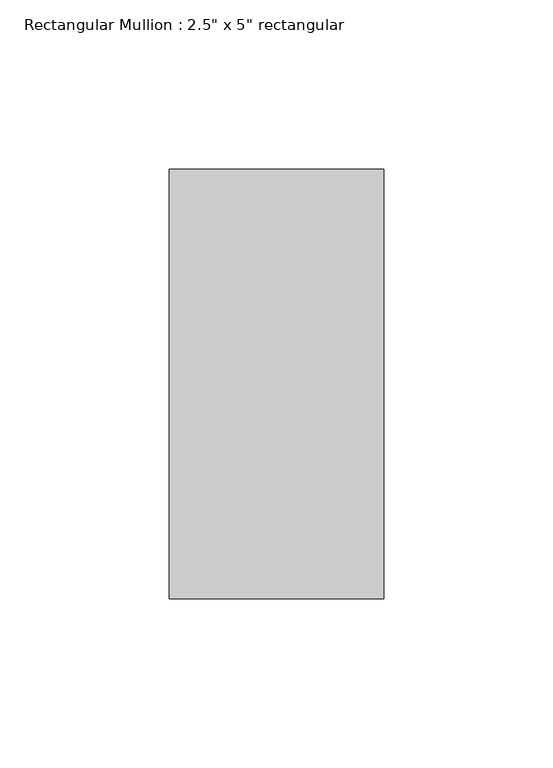
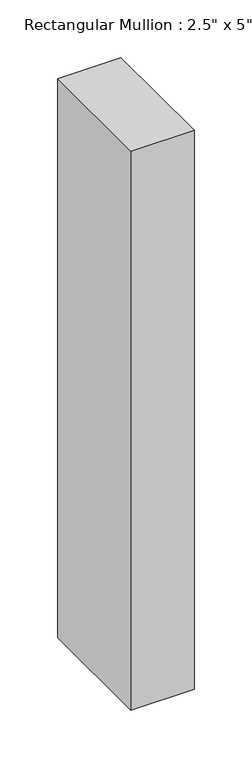
"""IFC4 building model written with IfcOpenShell, lengths in millimetres: member geometry."""

from ifc_helpers import new_model, si_unit, frame, origin, place, context, project, spatial, polyline, outline, extrude, source, transform, mapped, element, save


def member_f68a8c1e(model_context):
    return source(origin(), model_context, "Body", "SweptSolid", [
        extrude(outline(polyline([(0.0, 63.5), (0.0, -63.5), (-63.5, -63.5), (-63.5, 63.5), (0.0, 63.5)])), frame((0.0, 0.0, -592.655826), z_axis=(0.0, 0.0, 1.0), x_axis=(1.0, 0.0, 0.0)), (0.0, 0.0, 1.0), 592.655826),
    ])


if __name__ == "__main__":
    model = new_model("IFC4")
    model_context = context("Model", 3, world=origin())
    ifc_project = project(units=[si_unit("LENGTHUNIT", "METRE", prefix="MILLI")], contexts=[model_context])
    site = spatial("IfcSite", under=ifc_project)
    building = spatial("IfcBuilding", under=site)
    placement = place(None, origin())
    member_shape = member_f68a8c1e(model_context)
    element("IfcMember", 1, ObjectType="Rectangular Mullion : 2.5\" x 5\" rectangular", at=placement, inside=building, context=model_context, shape_type="MappedRepresentation", body=[
        mapped(member_shape, transform((0.0, 0.0, 0.0), x_axis=(1.0, 0.0, 0.0), y_axis=(0.0, 1.0, 0.0), z_axis=(0.0, 0.0, 1.0))),
    ])
    save(model, "model.ifc")

# Revit data of these elements
# Type "Rectangular Mullion : 2.5\" x 5\" rectangular"
#   built-in parameter 1007304 = 0.416667 (stored number, unit not read)
#   built-in parameter 1007301 = 0.104167 (stored number, unit not read)
#   built-in parameter 1007300 = 0.104167 (stored number, unit not read)
# Element 1 (IfcMember, "Rectangular Mullion : 2.5\" x 5\" rectangular")
#   Materials on its faces: "Aluminum"
# Materials
#   "Aluminum": class "Metal", colour RGB 247 247 247, transparency 0, Description = "Aluminum 6061", Cost = 0
